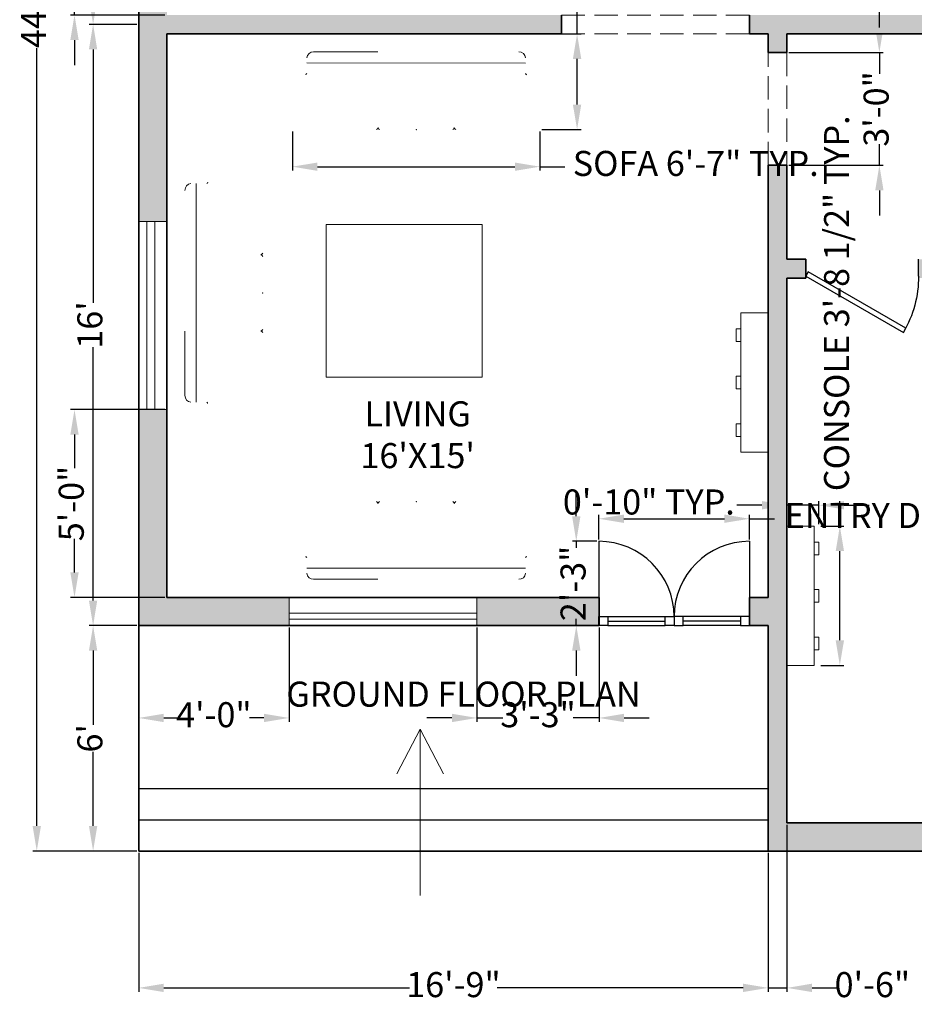
# Model space of a CAD drawing. Units: inches. Extents: x 2073 to 2646, y 2372 to 3017.
# Tile 1 of 8: x 2110 to 2396, y 2372 to 2686. Entities that reach past the tile are written whole.
import ezdxf

# ---------------------------------------------------------------- set-up
doc = ezdxf.new("R2010")
doc.units = ezdxf.units.IN
doc.linetypes.add('DASH', pattern=[0.35, 0.25, -0.1])
for name, color, linetype, lineweight in [('A-ANNO-DIMS', 2, 'Continuous', 18), ('A-ANNO-SYMB', 7, 'Continuous', 18), ('A-ANNO-TEXT', 7, 'Continuous', 25), ('A-AREA-IDEN', 7, 'Continuous', 25), ('A-DOOR', 3, 'Continuous', 25), ('A-FLOR-STRS', 7, 'Continuous', 25), ('A-FURN', 8, 'Continuous', 18), ('A-GLAZ', 4, 'Continuous', 18), ('A-WALL', 7, 'Continuous', 35), ('A-WALL-OVHD', 7, 'DASH', 18), ('A-WALL-PATT', 30, 'Continuous', 13)]:
    doc.layers.add(name, color=color, linetype=linetype, lineweight=lineweight)
doc.styles.get("Standard").update_dxf_attribs({"font": 'arial.ttf'})
doc.dimstyles.new('ISO-25', dxfattribs={"dimtxt": 8, "dimasz": 8, "dimexe": 1.25, "dimexo": 0.625, "dimtad": 0, "dimdec": 1, "dimlunit": 4, "dimtxsty": 'Standard', "dimcen": 2.5, "dimadec": 0, "dimazin": 0, "dimtfac": 1, "dimtdec": 1, "dimtmove": 0, "dimatfit": 3, "dimfxl": 1, "dimarcsym": 0})

# ---------------------------------------------------------------- blocks, each defined once
blk = doc.blocks.new('*D1')
at = {"layer": 'A-ANNO-DIMS', "color": 0, "lineweight": -2, "transparency": 16777216}
for p, q in [((2147.67, 2492.66), (2132.48, 2492.66)), ((2133.73, 2484.66), (2133.73, 2460.99)), ((2133.73, 2428.66), (2133.73, 2452.34)), ((2147.67, 2420.66), (2132.48, 2420.66))]:
    blk.add_line(p, q, dxfattribs=at)
at = {"layer": 'A-ANNO-DIMS', "color": 0, "transparency": 16777216}
for points in [[(2132.4, 2484.66), (2135.06, 2484.66), (2133.73, 2492.66)], [(2132.4, 2428.66), (2135.06, 2428.66), (2133.73, 2420.66)]]:
    blk.add_solid(points, dxfattribs=at)
at = {"layer": 'Defpoints', "color": 0, "transparency": 16777216}
for p in [(2133.73, 2492.66), (2148.29, 2492.66), (2148.29, 2420.66)]:
    blk.add_point(p, dxfattribs=at)
at = {"layer": 'A-ANNO-DIMS', "color": 0, "transparency": 16777216, "insert": (2133.73, 2456.66), "char_height": 8, "attachment_point": 5, "rotation": 90}
blk.add_mtext("6'", dxfattribs=at)
blk = doc.blocks.new('*D2')
at = {"layer": 'A-ANNO-DIMS', "color": 0, "lineweight": -2, "transparency": 16777216}
for p, q in [((2147.67, 2684.66), (2132.48, 2684.66)), ((2133.73, 2676.66), (2133.73, 2595.7)), ((2133.73, 2500.66), (2133.73, 2581.63)), ((2147.67, 2492.66), (2132.48, 2492.66))]:
    blk.add_line(p, q, dxfattribs=at)
at = {"layer": 'A-ANNO-DIMS', "color": 0, "transparency": 16777216}
for points in [[(2132.4, 2676.66), (2135.06, 2676.66), (2133.73, 2684.66)], [(2132.4, 2500.66), (2135.06, 2500.66), (2133.73, 2492.66)]]:
    blk.add_solid(points, dxfattribs=at)
at = {"layer": 'Defpoints', "color": 0, "transparency": 16777216}
for p in [(2133.73, 2684.66), (2148.29, 2684.66), (2148.29, 2492.66)]:
    blk.add_point(p, dxfattribs=at)
at = {"layer": 'A-ANNO-DIMS', "color": 0, "transparency": 16777216, "insert": (2133.73, 2588.66), "char_height": 8, "attachment_point": 5, "rotation": 90}
blk.add_mtext("16'", dxfattribs=at)
blk = doc.blocks.new('*D3')
at = {"layer": 'A-ANNO-DIMS', "color": 0, "lineweight": -2, "transparency": 16777216}
for p, q in [((2147.67, 2948.66), (2132.48, 2948.66)), ((2133.73, 2940.66), (2133.73, 2824.15)), ((2133.73, 2692.66), (2133.73, 2809.18)), ((2147.67, 2684.66), (2132.48, 2684.66))]:
    blk.add_line(p, q, dxfattribs=at)
at = {"layer": 'A-ANNO-DIMS', "color": 0, "transparency": 16777216}
for points in [[(2132.4, 2940.66), (2135.06, 2940.66), (2133.73, 2948.66)], [(2132.4, 2692.66), (2135.06, 2692.66), (2133.73, 2684.66)]]:
    blk.add_solid(points, dxfattribs=at)
at = {"layer": 'Defpoints', "color": 0, "transparency": 16777216}
for p in [(2133.73, 2948.66), (2148.29, 2948.66), (2148.29, 2684.66)]:
    blk.add_point(p, dxfattribs=at)
at = {"layer": 'A-ANNO-DIMS', "color": 0, "transparency": 16777216, "insert": (2133.73, 2816.66), "char_height": 8, "attachment_point": 5, "rotation": 90}
blk.add_mtext("22'", dxfattribs=at)
blk = doc.blocks.new('*D8')
at = {"layer": 'A-ANNO-DIMS', "color": 0, "lineweight": -2, "transparency": 16777216}
for p, q in [((2147.67, 2948.66), (2114.49, 2948.66)), ((2115.74, 2940.66), (2115.74, 2692.24)), ((2115.74, 2428.66), (2115.74, 2677.09)), ((2147.67, 2420.66), (2114.49, 2420.66))]:
    blk.add_line(p, q, dxfattribs=at)
at = {"layer": 'A-ANNO-DIMS', "color": 0, "transparency": 16777216}
for points in [[(2114.41, 2940.66), (2117.08, 2940.66), (2115.74, 2948.66)], [(2114.41, 2428.66), (2117.08, 2428.66), (2115.74, 2420.66)]]:
    blk.add_solid(points, dxfattribs=at)
at = {"layer": 'Defpoints', "color": 0, "transparency": 16777216}
for p in [(2148.29, 2948.66), (2115.74, 2420.66), (2148.29, 2420.66)]:
    blk.add_point(p, dxfattribs=at)
at = {"layer": 'A-ANNO-DIMS', "color": 0, "transparency": 16777216, "insert": (2115.74, 2684.66), "char_height": 8, "attachment_point": 5, "rotation": 90}
blk.add_mtext("44'", dxfattribs=at)
blk = doc.blocks.new('Clinicians and patient chairs 9_dwgmodels.com')
at = {"color": 0}
for points in [[(-907.9, 0, 0, 0, 0), (-959.6, -11.1, 4.62, 4.62, 0)], [(907.9, 0, 0, 0, 0), (-907.9, 0, 4.62, 4.62, 0)], [(959.6, -11.1, 0, 0, 0), (907.9, 0, 4.62, 4.62, 0)], [(-1015.6, -68.3, 0, 0, 0), (-1025.5, -106.3, 4.62, 4.62, 0)], [(-994.7, -35.9, 0, 0, 0), (-1015.6, -68.3, 4.62, 4.62, 0)], [(-959.6, -11.1, 0, 0, 0), (-994.7, -35.9, 4.62, 4.62, 0)], [(994.7, -35.9, 0, 0, 0), (959.6, -11.1, 4.62, 4.62, 0)], [(1015.6, -68.3, 0, 0, 0), (994.7, -35.9, 4.62, 4.62, 0)], [(1025.5, -106.3, 0, 0, 0), (1015.6, -68.3, 4.62, 4.62, 0)], [(-1025.5, -106.3, 0, 0, 0), (-1025.5, -779.5, 4.62, 4.62, 0)], [(-313.4, -149.9, 0, 0, 0), (-318.1, -149.9, 4.62, 4.62, 0)], [(-314.5, -150.4, 0, 0, 0), (-315.7, -159.3, 4.62, 4.62, 0)], [(-315.7, -159.3, 0, 0, 0), (-315.7, -777.3, 4.62, 4.62, 0)], [(-309.5, -148.3, 0, 0, 0), (-314.5, -150.4, 4.62, 4.62, 0)], [(-308, -148.3, 0, 0, 0), (-309.5, -148.3, 4.62, 4.62, 0)], [(-307.5, -148.3, 0, 0, 0), (-308, -148.3, 4.62, 4.62, 0)], [(242.9, -148.3, 0, 0, 0), (-307.5, -148.3, 4.62, 4.62, 0)], [(242.9, -148.3, 0, 0, 0), (296, -148.3, 4.62, 4.62, 0)], [(296, -148.3, 0, 0, 0), (307.5, -148.3, 4.62, 4.62, 0)], [(308, -148.3, 0, 0, 0), (307.5, -148.3, 4.62, 4.62, 0)], [(309.5, -148.3, 0, 0, 0), (308, -148.3, 4.62, 4.62, 0)], [(309.5, -148.3, 0, 0, 0), (314.5, -150.4, 4.62, 4.62, 0)], [(849.5, -149.9, 0, 0, 0), (313.4, -149.9, 4.62, 4.62, 0)], [(314.5, -150.4, 0, 0, 0), (315.7, -159.3, 4.62, 4.62, 0)], [(315.7, -159.3, 0, 0, 0), (315.7, -777.3, 4.62, 4.62, 0)], [(315.7, -161.8, 0, 0, 0), (315.7, -777.3, 4.62, 4.62, 0)], [(1025.5, -779.5, 0, 0, 0), (1025.5, -106.3, 4.62, 4.62, 0)], [(1025.5, -779.5, 0, 0, 0), (1025.5, -117.3, 4.62, 4.62, 0)], [(-906.6, -285, 0, 0, 0), (-906.4, -198.1, 4.62, 4.62, 0)], [(906.9, -327, 0, 0, 0), (906.4, -199.7, 4.62, 4.62, 0)], [(-906.8, -305.4, 0, 0, 0), (-906.9, -324.5, 4.62, 4.62, 0)], [(-906.9, -324.5, 0, 0, 0), (-906.9, -329.8, 4.62, 4.62, 0)], [(-906.6, -285, 0, 0, 0), (-906.8, -305.4, 4.62, 4.62, 0)], [(906.9, -327, 0, 0, 0), (906.9, -329.9, 4.62, 4.62, 0)], [(-1023, -329.7, 0, 0, 0), (-1019.2, -332.9, 4.62, 4.62, 0)], [(-1019.8, -340.2, 0, 0, 0), (-1023, -348.6, 4.62, 4.62, 0)], [(-1010.3, -335.9, 0, 0, 0), (-1019.8, -340.2, 4.62, 4.62, 0)], [(-1019.2, -332.9, 0, 0, 0), (-1019, -333, 4.62, 4.62, 0)], [(-1019, -333, 0, 0, 0), (-1018.9, -333.1, 4.62, 4.62, 0)], [(-1013.9, -334.2, 0, 0, 0), (-1018.9, -333.1, 4.62, 4.62, 0)], [(-1013.9, -334.2, 0, 0, 0), (-964.4, -335.7, 4.62, 4.62, 0)], [(-917.1, -337, 0, 0, 0), (-1010.3, -335.9, 4.62, 4.62, 0)], [(-964.4, -335.7, 0, 0, 0), (-927.1, -336.8, 4.62, 4.62, 0)], [(964.4, -335.7, 0, 0, 0), (914.9, -337.2, 4.62, 4.62, 0)], [(917.1, -339.4, 0, 0, 0), (1010.3, -338.4, 4.62, 4.62, 0)], [(1013.9, -334.2, 0, 0, 0), (964.4, -335.7, 4.62, 4.62, 0)], [(1010.3, -338.4, 0, 0, 0), (1019.8, -342.7, 4.62, 4.62, 0)], [(1013.9, -334.2, 0, 0, 0), (1018.9, -333.1, 4.62, 4.62, 0)], [(1018.9, -333.1, 0, 0, 0), (1019, -333, 4.62, 4.62, 0)], [(1019.2, -332.9, 0, 0, 0), (1019, -333, 4.62, 4.62, 0)], [(1023, -329.7, 0, 0, 0), (1019.2, -332.9, 4.62, 4.62, 0)], [(1019.8, -342.7, 0, 0, 0), (1023, -351.1, 4.62, 4.62, 0)], [(1023, -351.1, 0, 0, 0), (1022.6, -779.8, 4.62, 4.62, 0)], [(-1025.5, -779.5, 0, 0, 0), (-1022.2, -788.7, 4.62, 4.62, 0)], [(-1022.2, -788.7, 0, 0, 0), (-1021.6, -789.8, 4.62, 4.62, 0)], [(-1021.6, -789.8, 0, 0, 0), (-1020.6, -790.5, 4.62, 4.62, 0)], [(-1020.6, -790.5, 0, 0, 0), (-1013.6, -793.7, 4.62, 4.62, 0)], [(-1013.6, -793.7, 0, 0, 0), (1013.6, -793.7, 4.62, 4.62, 0)], [(1019.8, -788.8, 0, 0, 0), (1013.1, -793.7, 4.62, 4.62, 0)], [(1013.6, -793.7, 0, 0, 0), (1020.6, -790.5, 4.62, 4.62, 0)], [(1022.6, -779.8, 0, 0, 0), (1019.8, -788.8, 4.62, 4.62, 0)], [(1020.6, -790.5, 0, 0, 0), (1021.6, -789.8, 4.62, 4.62, 0)], [(1022.2, -788.7, 0, 0, 0), (1021.6, -789.8, 4.62, 4.62, 0)], [(1022.2, -788.7, 0, 0, 0), (1025.5, -779.5, 4.62, 4.62, 0)]]:
    blk.add_lwpolyline(points, format="xyseb", dxfattribs=at)
for points in [[(-849.5, -149.9), (-318.1, -149.9)], [(-906.5, -241.5), (906.5, -242.3)]]:
    blk.add_lwpolyline(points, dxfattribs=at)
for centre, radius, start, end in [((-851.7, -204.8), 54.9, 87.66794, 174.72556), ((851.7, -204.8), 54.9, 5.27444, 92.33206), ((-916.6, -326.8), 10.2, 267.54544, 342.40568), ((916.9, -329.4), 10, 182.60942, 270.79497), ((-337, -773.8), 21.5, 292.11503, 350.63044), ((-294.5, -773.8), 21.5, 189.36956, 247.88497), ((294.5, -773.8), 21.5, 292.11503, 350.63044), ((336.9, -773.8), 21.5, 189.36956, 247.88497)]:
    blk.add_arc(centre, radius, start, end, dxfattribs=at)
blk.add_point((0, -793.7), dxfattribs=at)
blk = doc.blocks.new('*U19')
for p, q in [((0, 0), (0, -6)), ((40, 0), (40, -6))]:
    blk.add_line(p, q)
blk.add_lwpolyline([(0, 0), (34.64, 20), (35.52, 18.48), (0.87, -1.52)], close=True)
blk.add_arc((0, 0), 40, 0, 30)
blk = doc.blocks.new('md')
for points in [[(1926.45, 2847.63), (1926.45, 2824.6)], [(1972.51, 2847.63), (1972.51, 2824.6)], [(1929.2, 2824.6), (1946.72, 2824.6)], [(1969.76, 2824.6), (1952.24, 2824.6)], [(1929.2, 2823.22), (1946.72, 2823.22)], [(1929.2, 2821.85), (1946.72, 2821.85)], [(1969.76, 2823.22), (1952.24, 2823.22)], [(1969.76, 2821.85), (1952.24, 2821.85)]]:
    blk.add_lwpolyline(points)
for points in [[(1926.45, 2824.6), (1929.2, 2824.6), (1929.2, 2821.85), (1926.45, 2821.85)], [(1946.72, 2824.6), (1949.48, 2824.6), (1949.48, 2821.85), (1946.72, 2821.85)], [(1946.72, 2824.6), (1949.48, 2824.6), (1949.48, 2821.85), (1946.72, 2821.85)], [(1952.24, 2824.6), (1949.48, 2824.6), (1949.48, 2821.85), (1952.24, 2821.85)], [(1972.51, 2824.6), (1969.76, 2824.6), (1969.76, 2821.85), (1972.51, 2821.85)]]:
    blk.add_lwpolyline(points, close=True)
for centre, start, end in [((1926.45, 2824.6), 0, 90), ((1972.51, 2824.6), 90, 180)]:
    blk.add_arc(centre, 23.03, start, end)
blk = doc.blocks.new('GLAZ-60IN')
for p, q in [((0, 60), (0, 0)), ((2.6, 60), (2.6, 0))]:
    blk.add_line(p, q)
blk = doc.blocks.new('WALL-CONSOLE-44IN')
for points in [[(10.22, 44.47), (1.5, 44.47), (1.5, 0), (10.22, 0)], [(1.5, 39.34), (0, 39.34), (0, 35.33), (1.5, 35.33)], [(1.5, 24.24), (0, 24.24), (0, 20.23), (1.5, 20.23)], [(1.5, 8.99), (0, 8.99), (0, 4.98), (1.5, 4.98)]]:
    blk.add_lwpolyline(points, close=True)
blk = doc.blocks.new('*D29')
at = {"layer": 'A-ANNO-DIMS', "color": 0, "lineweight": -2, "transparency": 16777216}
for p, q in [((2372.17, 2524.43), (2372.17, 2532.43)), ((2366.13, 2524.43), (2373.42, 2524.43)), ((2372.17, 2487.96), (2372.17, 2516.43)), ((2366.13, 2479.96), (2373.42, 2479.96))]:
    blk.add_line(p, q, dxfattribs=at)
at = {"layer": 'A-ANNO-DIMS', "color": 0, "transparency": 16777216}
for points in [[(2370.84, 2516.43), (2373.51, 2516.43), (2372.17, 2524.43)], [(2370.84, 2487.96), (2373.51, 2487.96), (2372.17, 2479.96)]]:
    blk.add_solid(points, dxfattribs=at)
at = {"layer": 'Defpoints', "color": 0, "transparency": 16777216}
for p in [(2365.5, 2524.43), (2372.17, 2524.43), (2365.5, 2479.96)]:
    blk.add_point(p, dxfattribs=at)
at = {"layer": 'A-ANNO-DIMS', "color": 0, "transparency": 16777216, "insert": (2372.17, 2595.59), "char_height": 8, "attachment_point": 5, "rotation": 90}
blk.add_mtext('CONSOLE 3\'-8 1/2" TYP.', dxfattribs=at)
blk = doc.blocks.new('*D30')
at = {"layer": 'A-ANNO-DIMS', "color": 0, "lineweight": -2, "transparency": 16777216}
for p, q in [((2355.29, 2525.05), (2355.29, 2532.35)), ((2365.5, 2525.05), (2365.5, 2532.35)), ((2347.29, 2531.1), (2339.29, 2531.1)), ((2365.5, 2531.1), (2355.29, 2531.1)), ((2373.5, 2531.1), (2381.5, 2531.1))]:
    blk.add_line(p, q, dxfattribs=at)
at = {"layer": 'A-ANNO-DIMS', "color": 0, "transparency": 16777216}
for points in [[(2347.29, 2532.43), (2347.29, 2529.77), (2355.29, 2531.1)], [(2373.5, 2532.43), (2373.5, 2529.77), (2365.5, 2531.1)]]:
    blk.add_solid(points, dxfattribs=at)
at = {"layer": 'Defpoints', "color": 0, "transparency": 16777216}
for p in [(2355.29, 2531.1), (2355.29, 2524.43), (2365.5, 2524.43)]:
    blk.add_point(p, dxfattribs=at)
at = {"layer": 'A-ANNO-DIMS', "color": 0, "transparency": 16777216, "insert": (2311.18, 2531.1), "char_height": 8, "attachment_point": 5}
blk.add_mtext('0\'-10" TYP.', dxfattribs=at)
blk = doc.blocks.new('*D31')
at = {"layer": 'A-ANNO-DIMS', "color": 0, "lineweight": -2, "transparency": 16777216}
for p, q in [((2197.36, 2650.45), (2197.36, 2637.97)), ((2276.41, 2650.45), (2276.41, 2637.97)), ((2205.36, 2639.22), (2268.41, 2639.22)), ((2276.41, 2639.22), (2284.41, 2639.22))]:
    blk.add_line(p, q, dxfattribs=at)
at = {"layer": 'A-ANNO-DIMS', "color": 0, "transparency": 16777216}
for points in [[(2205.36, 2640.55), (2205.36, 2637.88), (2197.36, 2639.22)], [(2268.41, 2640.55), (2268.41, 2637.88), (2276.41, 2639.22)]]:
    blk.add_solid(points, dxfattribs=at)
at = {"layer": 'Defpoints', "color": 0, "transparency": 16777216}
for p in [(2197.36, 2651.07), (2276.41, 2651.07), (2276.41, 2639.22)]:
    blk.add_point(p, dxfattribs=at)
at = {"layer": 'A-ANNO-DIMS', "color": 0, "transparency": 16777216, "insert": (2326.16, 2639.22), "char_height": 8, "attachment_point": 5}
blk.add_mtext('SOFA 6\'-7" TYP.', dxfattribs=at)
blk = doc.blocks.new('*D32')
at = {"layer": 'A-ANNO-DIMS', "color": 0, "lineweight": -2, "transparency": 16777216}
for p, q in [((2288.27, 2681.66), (2288.27, 2689.66)), ((2277.03, 2681.66), (2289.52, 2681.66)), ((2288.27, 2659.07), (2288.27, 2673.66)), ((2277.03, 2651.07), (2289.52, 2651.07))]:
    blk.add_line(p, q, dxfattribs=at)
at = {"layer": 'A-ANNO-DIMS', "color": 0, "transparency": 16777216}
for points in [[(2286.93, 2673.66), (2289.6, 2673.66), (2288.27, 2681.66)], [(2286.93, 2659.07), (2289.6, 2659.07), (2288.27, 2651.07)]]:
    blk.add_solid(points, dxfattribs=at)
at = {"layer": 'Defpoints', "color": 0, "transparency": 16777216}
for p in [(2276.41, 2681.66), (2288.27, 2681.66), (2276.41, 2651.07)]:
    blk.add_point(p, dxfattribs=at)
at = {"layer": 'A-ANNO-DIMS', "color": 0, "transparency": 16777216, "insert": (2288.27, 2724.06), "char_height": 8, "attachment_point": 5, "rotation": 90}
blk.add_mtext('2\'-6 1/2" TYP.', dxfattribs=at)
blk = doc.blocks.new('*D41')
at = {"layer": 'A-ANNO-DIMS', "color": 0, "lineweight": -2, "transparency": 16777216}
for p, q in [((2295.23, 2520.2), (2295.23, 2528.03)), ((2303.23, 2526.78), (2335.29, 2526.78)), ((2343.29, 2520.2), (2343.29, 2528.03)), ((2343.29, 2526.78), (2351.29, 2526.78))]:
    blk.add_line(p, q, dxfattribs=at)
at = {"layer": 'A-ANNO-DIMS', "color": 0, "transparency": 16777216}
for points in [[(2303.23, 2528.12), (2303.23, 2525.45), (2295.23, 2526.78)], [(2335.29, 2528.12), (2335.29, 2525.45), (2343.29, 2526.78)]]:
    blk.add_solid(points, dxfattribs=at)
at = {"layer": 'Defpoints', "color": 0, "transparency": 16777216}
for p in [(2343.29, 2526.78), (2295.23, 2519.57), (2343.29, 2519.57)]:
    blk.add_point(p, dxfattribs=at)
at = {"layer": 'A-ANNO-DIMS', "color": 0, "transparency": 16777216, "insert": (2401.15, 2526.78), "char_height": 8, "attachment_point": 5}
blk.add_mtext('ENTRY DOOR 4\'-0"', dxfattribs=at)
blk = doc.blocks.new('*D42')
at = {"layer": 'A-ANNO-DIMS', "color": 0, "lineweight": -2, "transparency": 16777216}
for p, q in [((2288.02, 2527.57), (2288.02, 2535.57)), ((2294.6, 2519.57), (2286.77, 2519.57)), ((2288.02, 2519.57), (2288.02, 2517.44)), ((2288.02, 2492.66), (2288.02, 2494.79)), ((2294.6, 2492.66), (2286.77, 2492.66)), ((2288.02, 2484.66), (2288.02, 2476.66))]:
    blk.add_line(p, q, dxfattribs=at)
at = {"layer": 'A-ANNO-DIMS', "color": 0, "transparency": 16777216}
for points in [[(2286.68, 2527.57), (2289.35, 2527.57), (2288.02, 2519.57)], [(2286.68, 2484.66), (2289.35, 2484.66), (2288.02, 2492.66)]]:
    blk.add_solid(points, dxfattribs=at)
at = {"layer": 'Defpoints', "color": 0, "transparency": 16777216}
for p in [(2288.02, 2519.57), (2295.23, 2519.57), (2295.23, 2492.66)]:
    blk.add_point(p, dxfattribs=at)
at = {"layer": 'A-ANNO-DIMS', "color": 0, "transparency": 16777216, "insert": (2288.02, 2506.12), "char_height": 8, "attachment_point": 5, "rotation": 90}
blk.add_mtext('2\'-3"', dxfattribs=at)
blk = doc.blocks.new('*D43')
at = {"layer": 'A-ANNO-DIMS', "color": 0, "lineweight": -2, "transparency": 16777216}
for p, q in [((2148.29, 2420.04), (2148.29, 2375.7)), ((2349.29, 2420.04), (2349.29, 2375.7)), ((2156.29, 2376.95), (2234.8, 2376.95)), ((2341.29, 2376.95), (2262.78, 2376.95))]:
    blk.add_line(p, q, dxfattribs=at)
at = {"layer": 'A-ANNO-DIMS', "color": 0, "transparency": 16777216}
for points in [[(2156.29, 2378.29), (2156.29, 2375.62), (2148.29, 2376.95)], [(2341.29, 2378.29), (2341.29, 2375.62), (2349.29, 2376.95)]]:
    blk.add_solid(points, dxfattribs=at)
at = {"layer": 'Defpoints', "color": 0, "transparency": 16777216}
for p in [(2148.29, 2420.66), (2349.29, 2420.66), (2349.29, 2376.95)]:
    blk.add_point(p, dxfattribs=at)
at = {"layer": 'A-ANNO-DIMS', "color": 0, "transparency": 16777216, "insert": (2248.79, 2376.95), "char_height": 8, "attachment_point": 5}
blk.add_mtext('16\'-9"', dxfattribs=at)
blk = doc.blocks.new('*D47')
at = {"layer": 'A-ANNO-DIMS', "color": 0, "lineweight": -2, "transparency": 16777216}
for p, q in [((2355.29, 2429.04), (2355.29, 2375.7)), ((2349.29, 2420.04), (2349.29, 2375.7)), ((2341.29, 2376.95), (2333.29, 2376.95)), ((2349.29, 2376.95), (2355.29, 2376.95)), ((2363.29, 2376.95), (2371.29, 2376.95))]:
    blk.add_line(p, q, dxfattribs=at)
at = {"layer": 'A-ANNO-DIMS', "color": 0, "transparency": 16777216}
for points in [[(2341.29, 2378.29), (2341.29, 2375.62), (2349.29, 2376.95)], [(2363.29, 2378.29), (2363.29, 2375.62), (2355.29, 2376.95)]]:
    blk.add_solid(points, dxfattribs=at)
at = {"layer": 'Defpoints', "color": 0, "transparency": 16777216}
for p in [(2355.29, 2429.66), (2349.29, 2420.66), (2355.29, 2376.95)]:
    blk.add_point(p, dxfattribs=at)
at = {"layer": 'A-ANNO-DIMS', "color": 0, "transparency": 16777216, "insert": (2382.55, 2376.95), "char_height": 8, "attachment_point": 5}
blk.add_mtext('0\'-6"', dxfattribs=at)
blk = doc.blocks.new('*D48')
at = {"layer": 'A-ANNO-DIMS', "color": 0, "lineweight": -2, "transparency": 16777216}
for p, q in [((2148.29, 2492.04), (2148.29, 2461.91)), ((2196.29, 2492.04), (2196.29, 2461.91)), ((2156.29, 2463.16), (2160.87, 2463.16)), ((2188.29, 2463.16), (2183.71, 2463.16))]:
    blk.add_line(p, q, dxfattribs=at)
at = {"layer": 'A-ANNO-DIMS', "color": 0, "transparency": 16777216}
for points in [[(2156.29, 2464.5), (2156.29, 2461.83), (2148.29, 2463.16)], [(2188.29, 2464.5), (2188.29, 2461.83), (2196.29, 2463.16)]]:
    blk.add_solid(points, dxfattribs=at)
at = {"layer": 'Defpoints', "color": 0, "transparency": 16777216}
for p in [(2148.29, 2492.66), (2196.29, 2492.66), (2148.29, 2463.16)]:
    blk.add_point(p, dxfattribs=at)
at = {"layer": 'A-ANNO-DIMS', "color": 0, "transparency": 16777216, "insert": (2172.29, 2463.16), "char_height": 8, "attachment_point": 5}
blk.add_mtext('4\'-0"', dxfattribs=at)
blk = doc.blocks.new('*D49')
at = {"layer": 'A-ANNO-DIMS', "color": 0, "lineweight": -2, "transparency": 16777216}
for p, q in [((2256.29, 2492.04), (2256.29, 2461.91)), ((2295.29, 2492.04), (2295.29, 2461.91)), ((2248.29, 2463.16), (2240.29, 2463.16)), ((2256.29, 2463.16), (2264.53, 2463.16)), ((2295.29, 2463.16), (2287.05, 2463.16)), ((2303.29, 2463.16), (2311.29, 2463.16))]:
    blk.add_line(p, q, dxfattribs=at)
at = {"layer": 'A-ANNO-DIMS', "color": 0, "transparency": 16777216}
for points in [[(2248.29, 2464.5), (2248.29, 2461.83), (2256.29, 2463.16)], [(2303.29, 2464.5), (2303.29, 2461.83), (2295.29, 2463.16)]]:
    blk.add_solid(points, dxfattribs=at)
at = {"layer": 'Defpoints', "color": 0, "transparency": 16777216}
for p in [(2256.29, 2492.66), (2295.29, 2492.66), (2256.29, 2463.16)]:
    blk.add_point(p, dxfattribs=at)
at = {"layer": 'A-ANNO-DIMS', "color": 0, "transparency": 16777216, "insert": (2275.79, 2463.16), "char_height": 8, "attachment_point": 5}
blk.add_mtext('3\'-3"', dxfattribs=at)
blk = doc.blocks.new('*D53')
at = {"layer": 'A-ANNO-DIMS', "color": 0, "lineweight": -2, "transparency": 16777216}
for p, q in [((2384.79, 2683.66), (2384.79, 2691.66)), ((2355.92, 2675.66), (2386.04, 2675.66)), ((2384.79, 2675.66), (2384.79, 2668.92)), ((2384.79, 2639.66), (2384.79, 2646.41)), ((2355.92, 2639.66), (2386.04, 2639.66)), ((2384.79, 2631.66), (2384.79, 2623.66))]:
    blk.add_line(p, q, dxfattribs=at)
at = {"layer": 'A-ANNO-DIMS', "color": 0, "transparency": 16777216}
for points in [[(2383.46, 2683.66), (2386.12, 2683.66), (2384.79, 2675.66)], [(2383.46, 2631.66), (2386.12, 2631.66), (2384.79, 2639.66)]]:
    blk.add_solid(points, dxfattribs=at)
at = {"layer": 'Defpoints', "color": 0, "transparency": 16777216}
for p in [(2355.29, 2675.66), (2355.29, 2639.66), (2384.79, 2639.66)]:
    blk.add_point(p, dxfattribs=at)
at = {"layer": 'A-ANNO-DIMS', "color": 0, "transparency": 16777216, "insert": (2384.79, 2657.66), "char_height": 8, "attachment_point": 5, "rotation": 90}
blk.add_mtext('3\'-0"', dxfattribs=at)
blk = doc.blocks.new('*D59')
at = {"layer": 'A-ANNO-DIMS', "color": 0, "lineweight": -2, "transparency": 16777216}
for p, q in [((2156.67, 2561.66), (2126.54, 2561.66)), ((2127.79, 2553.66), (2127.79, 2542.92)), ((2127.79, 2509.66), (2127.79, 2520.41)), ((2156.67, 2501.66), (2126.54, 2501.66))]:
    blk.add_line(p, q, dxfattribs=at)
at = {"layer": 'A-ANNO-DIMS', "color": 0, "transparency": 16777216}
for points in [[(2126.46, 2553.66), (2129.12, 2553.66), (2127.79, 2561.66)], [(2126.46, 2509.66), (2129.12, 2509.66), (2127.79, 2501.66)]]:
    blk.add_solid(points, dxfattribs=at)
at = {"layer": 'Defpoints', "color": 0, "transparency": 16777216}
for p in [(2127.79, 2561.66), (2157.29, 2561.66), (2157.29, 2501.66)]:
    blk.add_point(p, dxfattribs=at)
at = {"layer": 'A-ANNO-DIMS', "color": 0, "transparency": 16777216, "insert": (2127.79, 2531.66), "char_height": 8, "attachment_point": 5, "rotation": 90}
blk.add_mtext('5\'-0"', dxfattribs=at)
blk = doc.blocks.new('*D60')
at = {"layer": 'A-ANNO-DIMS', "color": 0, "lineweight": -2, "transparency": 16777216}
for p, q in [((2127.79, 2712.25), (2127.79, 2720.25)), ((2156.67, 2704.25), (2126.54, 2704.25)), ((2127.79, 2687.66), (2127.79, 2704.25)), ((2156.67, 2687.66), (2126.54, 2687.66)), ((2127.79, 2679.66), (2127.79, 2671.66))]:
    blk.add_line(p, q, dxfattribs=at)
at = {"layer": 'A-ANNO-DIMS', "color": 0, "transparency": 16777216}
for points in [[(2126.46, 2712.25), (2129.12, 2712.25), (2127.79, 2704.25)], [(2126.46, 2679.66), (2129.12, 2679.66), (2127.79, 2687.66)]]:
    blk.add_solid(points, dxfattribs=at)
at = {"layer": 'Defpoints', "color": 0, "transparency": 16777216}
for p in [(2127.79, 2704.25), (2157.29, 2704.25), (2157.29, 2687.66)]:
    blk.add_point(p, dxfattribs=at)
at = {"layer": 'A-ANNO-DIMS', "color": 0, "transparency": 16777216, "insert": (2127.79, 2740.45), "char_height": 8, "attachment_point": 5, "rotation": 90}
blk.add_mtext('1\'-4 1/2"', dxfattribs=at)

msp = doc.modelspace()

# ---------------------------------------------------------------- hatches: boundary and pattern name
at = {"layer": 'A-WALL-PATT'}
h = msp.add_hatch(color=256, dxfattribs=at)
h.dxf.hatch_style = 1
h.paths.add_polyline_path([(2340.29, 2948.66), (2148.29, 2948.66), (2148.29, 2924.66), (2157.29, 2924.66), (2157.29, 2939.66), (2313.29, 2939.66), (2313.29, 2885.66), (2307.29, 2885.66), (2307.29, 2879.66), (2313.29, 2879.66), (2313.29, 2777.66), (2319.29, 2777.66), (2319.29, 2831.66), (2385.29, 2831.66), (2385.29, 2825.68), (2390.69, 2825.68, -0.004149), (2391.29, 2825.68), (2391.29, 2843.66), (2385.29, 2843.66), (2385.29, 2837.66), (2319.29, 2837.66), (2319.29, 2939.66), (2340.29, 2939.66)])
h.paths.add_polyline_path([(2271.29, 2885.66), (2157.29, 2885.66), (2157.29, 2900.66), (2148.29, 2900.66), (2148.29, 2856.74), (2157.29, 2856.74), (2157.29, 2879.66), (2271.29, 2879.66)], flags=17)
h.paths.add_polyline_path([(2157.29, 2796.74), (2148.29, 2796.74), (2148.29, 2764.25), (2157.29, 2764.25)])
h.paths.add_polyline_path([(2157.29, 2681.66), (2283.29, 2681.66), (2283.29, 2687.66), (2157.29, 2687.66), (2157.29, 2704.25), (2148.29, 2704.25), (2148.29, 2621.66), (2157.29, 2621.66)])
h.paths.add_polyline_path([(2196.29, 2501.66), (2157.29, 2501.66), (2157.29, 2561.66), (2148.29, 2561.66), (2148.29, 2492.66), (2196.29, 2492.66)])
h.paths.add_polyline_path([(2295.23, 2495.54), (2295.23, 2501.66), (2256.29, 2501.66), (2256.29, 2492.66), (2295.23, 2492.66)])
h.paths.add_polyline_path([(2355.29, 2603.66), (2361.29, 2603.66), (2361.29, 2609.66), (2355.29, 2609.66), (2355.29, 2639.66), (2349.29, 2639.66), (2349.29, 2501.66), (2343.29, 2501.66), (2343.29, 2492.66), (2349.29, 2492.66), (2349.29, 2420.66), (2532.29, 2420.66), (2532.29, 2486.66), (2523.29, 2486.66), (2523.29, 2429.66), (2355.29, 2429.66)])
h.paths.add_polyline_path([(2532.29, 2633.66), (2523.29, 2633.66), (2523.29, 2609.66), (2439.29, 2609.66), (2439.29, 2615.66), (2433.29, 2615.66), (2433.29, 2609.66), (2397.31, 2609.66), (2397.31, 2604.26, -0.004149), (2397.3, 2603.66), (2523.29, 2603.66), (2523.29, 2546.66), (2532.29, 2546.66)], flags=17)
h.paths.add_polyline_path([(2532.29, 2702.66), (2523.29, 2702.66), (2523.29, 2687.66), (2385.29, 2687.66), (2343.29, 2687.66), (2343.29, 2681.66), (2349.29, 2681.66), (2349.29, 2675.66), (2355.29, 2675.66), (2355.29, 2681.66), (2433.29, 2681.66), (2433.29, 2645.66), (2439.29, 2645.66), (2439.29, 2681.66), (2523.29, 2681.66), (2523.29, 2657.66), (2532.29, 2657.66)])
h.paths.add_polyline_path([(2532.29, 2831.66), (2523.29, 2831.66), (2523.29, 2783.66), (2391.29, 2783.66), (2391.29, 2789.66), (2385.29, 2789.66), (2385.29, 2777.66), (2523.29, 2777.66), (2523.29, 2762.66), (2532.29, 2762.66)])
h.paths.add_polyline_path([(2532.29, 2948.66), (2364.29, 2948.66), (2364.29, 2939.66), (2385.29, 2939.66), (2385.29, 2873.66), (2391.29, 2873.66), (2391.29, 2939.66), (2523.29, 2939.66), (2523.29, 2891.66), (2532.29, 2891.66)])

# ---------------------------------------------------------------- linework, layer by layer
at = {"layer": 'A-ANNO-SYMB'}
for p, q in [((2238.15, 2459.56), (2230.68, 2445.29)), ((2238.15, 2406.45), (2238.15, 2459.56)), ((2238.15, 2459.56), (2245.62, 2445.29))]:
    msp.add_line(p, q, dxfattribs=at)
at = {"layer": 'A-FLOR-STRS'}
for p, q in [((2148.29, 2440.66), (2349.29, 2440.66)), ((2148.29, 2430.66), (2349.29, 2430.66))]:
    msp.add_line(p, q, dxfattribs=at)
at = {"layer": 'A-FURN'}
msp.add_lwpolyline([(2208.2, 2620.73), (2257.95, 2620.73), (2257.95, 2572.02), (2208.2, 2572.02)], close=True, dxfattribs=at)
at = {"layer": 'A-GLAZ'}
for p, q in [((2157.29, 2621.66), (2148.29, 2621.66)), ((2157.29, 2561.66), (2148.29, 2561.66)), ((2196.29, 2501.66), (2196.29, 2492.66)), ((2256.29, 2501.66), (2256.29, 2492.66)), ((2196.29, 2496.66), (2256.29, 2496.66)), ((2196.29, 2494.66), (2256.29, 2494.66))]:
    msp.add_line(p, q, dxfattribs=at)
at = {"layer": 'A-WALL'}
for p, q in [((2148.29, 2948.66), (2148.29, 2420.66)), ((2283.29, 2687.66), (2283.29, 2681.66)), ((2343.29, 2687.66), (2343.29, 2681.66)), ((2157.29, 2681.66), (2283.29, 2681.66)), ((2157.29, 2681.66), (2157.29, 2501.66)), ((2343.29, 2681.66), (2349.29, 2681.66)), ((2349.29, 2681.66), (2349.29, 2675.66)), ((2355.29, 2681.66), (2355.29, 2675.66)), ((2355.29, 2681.66), (2433.29, 2681.66)), ((2349.29, 2675.66), (2355.29, 2675.66)), ((2349.29, 2639.66), (2355.29, 2639.66)), ((2349.29, 2639.66), (2349.29, 2501.66)), ((2355.29, 2639.66), (2355.29, 2609.66)), ((2355.29, 2609.66), (2361.29, 2609.66)), ((2361.29, 2609.66), (2361.29, 2603.66)), ((2355.29, 2603.66), (2361.29, 2603.66)), ((2355.29, 2429.66), (2355.29, 2603.66)), ((2157.29, 2501.66), (2295.29, 2501.66)), ((2295.29, 2501.66), (2295.29, 2492.66)), ((2343.29, 2501.66), (2343.29, 2492.66)), ((2343.29, 2501.66), (2349.29, 2501.66)), ((2148.29, 2492.66), (2295.29, 2492.66)), ((2343.29, 2492.66), (2349.29, 2492.66)), ((2349.29, 2492.66), (2349.29, 2420.66)), ((2355.29, 2429.66), (2523.29, 2429.66)), ((2148.29, 2420.66), (2532.29, 2420.66))]:
    msp.add_line(p, q, dxfattribs=at)
at = {"layer": 'A-WALL-OVHD', "ltscale": 30}
for points in [[(2283.29, 2687.66), (2343.29, 2687.66), (2343.29, 2681.66), (2283.29, 2681.66)], [(2349.29, 2675.66), (2355.29, 2675.66), (2355.29, 2639.66), (2349.29, 2639.66)]]:
    msp.add_lwpolyline(points, close=True, dxfattribs=at)

# ---------------------------------------------------------------- block references
at = {"layer": 'A-DOOR', "xscale": -0.90038727397209, "yscale": 0.90038727397209, "zscale": 0.90038727397209, "rotation": 180}
msp.add_blockref('*U19', (2361.29, 2604.26), dxfattribs=at)
at = {"layer": 'A-DOOR', "xscale": 1.043429121125784, "yscale": 1.043429121125784, "zscale": 1.043429121125784}
msp.add_blockref('md', (285.11, -451.73), dxfattribs=at)
at = {"layer": 'A-FURN', "xscale": 0.0385401032590329, "yscale": 0.0385401032590329, "zscale": 0.0385401032590329}
msp.add_blockref('Clinicians and patient chairs 9_dwgmodels.com', (2236.89, 2681.66), dxfattribs=at)
at = {"layer": 'A-FURN', "yscale": 0.0385401032590329, "zscale": 0.0385401032590329}
for p, xscale, rotation in [((2157.29, 2598.91), 0.0385401032590329, 90), ((2236.89, 2501.66), -0.0385401032590329, 180)]:
    msp.add_blockref('Clinicians and patient chairs 9_dwgmodels.com', p, dxfattribs=dict(at, xscale=xscale, rotation=rotation))
at = {"layer": 'A-FURN'}
msp.add_blockref('WALL-CONSOLE-44IN', (2339.07, 2548.07), dxfattribs=at)
at = {"layer": 'A-FURN', "extrusion": (0, 0, -1), "zscale": -1}
msp.add_blockref('WALL-CONSOLE-44IN', (-2365.51, 2479.96), dxfattribs=at)
at = {"layer": 'A-GLAZ'}
msp.add_blockref('GLAZ-60IN', (2150.89, 2561.66), dxfattribs=at)

# ---------------------------------------------------------------- texts
at = {"layer": 'A-ANNO-TEXT', "insert": (2182.04, 2474.77), "char_height": 8, "attachment_point": 1}
msp.add_mtext_dynamic_manual_height_columns('\\pxqc;GROUND FLOOR PLAN', width=139.927, gutter_width=12.5, heights=[0], dxfattribs=at)
at = {"layer": 'A-AREA-IDEN', "insert": (2200.28, 2564.28), "char_height": 8, "attachment_point": 1}
msp.add_mtext_dynamic_manual_height_columns("\\pxqc;LIVING\\P16'X15'", width=74.1792, gutter_width=12.5, heights=[0], dxfattribs=at)

# ---------------------------------------------------------------- dimensions: what is measured, and where the dimension line sits
at = {"layer": 'A-ANNO-DIMS'}
for base, p1, p2, angle, override, picture, middle in [((2115.74, 2420.66), (2148.29, 2948.66), (2148.29, 2420.66), 90, {"dimclrd": 0, "dimclre": 0, "dimclrt": 0}, '*D8', (2115.74, 2684.66)), ((2133.73, 2948.66), (2148.29, 2684.66), (2148.29, 2948.66), 90, {"dimclrd": 0, "dimclre": 0, "dimclrt": 0}, '*D3', (2133.73, 2816.66)), ((2127.79, 2704.25), (2157.29, 2687.66), (2157.29, 2704.25), 90, {"dimdec": 1, "dimlfac": 1, "dimrnd": 0, "dimzin": 1, "dimdsep": 46, "dimlunit": 4, "dimfrac": 2}, '*D60', (2127.79, 2740.45)), ((2384.79, 2639.66), (2355.29, 2675.66), (2355.29, 2639.66), 270, {"dimdec": 1, "dimlfac": 1, "dimrnd": 0, "dimzin": 1, "dimdsep": 46, "dimlunit": 4, "dimfrac": 2}, '*D53', (2384.79, 2657.66)), ((2133.73, 2684.66), (2148.29, 2492.66), (2148.29, 2684.66), 90, {"dimclrd": 0, "dimclre": 0, "dimclrt": 0}, '*D2', (2133.73, 2588.66)), ((2127.79, 2561.66), (2157.29, 2501.66), (2157.29, 2561.66), 90, {"dimdec": 1, "dimlfac": 1, "dimrnd": 0, "dimzin": 1, "dimdsep": 46, "dimlunit": 4, "dimfrac": 2}, '*D59', (2127.79, 2531.66)), ((2288.02, 2519.57), (2295.23, 2492.66), (2295.23, 2519.57), 90, {"dimdec": 1, "dimlfac": 1, "dimrnd": 0, "dimzin": 1, "dimdsep": 46, "dimlunit": 4, "dimfrac": 2}, '*D42', (2288.02, 2506.12)), ((2133.73, 2492.66), (2148.29, 2420.66), (2148.29, 2492.66), 90, {"dimclrd": 0, "dimclre": 0, "dimclrt": 0}, '*D1', (2133.73, 2456.66)), ((2148.29, 2463.16), (2196.29, 2492.66), (2148.29, 2492.66), 180, {"dimdec": 1, "dimlfac": 1, "dimrnd": 0, "dimzin": 1, "dimdsep": 46, "dimlunit": 4, "dimfrac": 2}, '*D48', (2172.29, 2463.16)), ((2256.29, 2463.16), (2295.29, 2492.66), (2256.29, 2492.66), 180, {"dimdec": 1, "dimlfac": 1, "dimrnd": 0, "dimzin": 1, "dimdsep": 46, "dimlunit": 4, "dimfrac": 2}, '*D49', (2275.79, 2463.16))]:
    dim = msp.add_linear_dim(base=base, p1=p1, p2=p2, angle=angle, dimstyle='ISO-25', override=override, dxfattribs=at)
    dim.commit()
    dim.dimension.update_dxf_attribs({"geometry": picture, "text_midpoint": middle})
for base, p1, p2, angle, text, picture, middle in [((2288.27, 2681.66), (2276.41, 2651.07), (2276.41, 2681.66), 90, '<> TYP.', '*D32', (2288.27, 2724.06)), ((2372.17, 2524.43), (2365.5, 2479.96), (2365.5, 2524.43), 90, 'CONSOLE <> TYP.', '*D29', (2372.17, 2595.59)), ((2355.29, 2531.1), (2365.5, 2524.43), (2355.29, 2524.43), 180, '<> TYP.', '*D30', (2311.18, 2531.1))]:
    dim = msp.add_linear_dim(base=base, p1=p1, p2=p2, angle=angle, text=text, dimstyle='ISO-25', override={"dimdec": 1, "dimlfac": 1, "dimrnd": 0, "dimzin": 1, "dimdsep": 46, "dimlunit": 4, "dimfrac": 2}, dxfattribs=at)
    dim.commit()
    dim.dimension.update_dxf_attribs({"geometry": picture, "text_midpoint": middle})
for base, p1, p2, text, picture, middle in [((2276.4094, 2639.2171), (2197.3622, 2651.0742), (2276.4094, 2651.0742), 'SOFA <> TYP.', '*D31', (2326.164, 2639.2171)), ((2343.29, 2526.78), (2295.23, 2519.57), (2343.29, 2519.57), 'ENTRY DOOR <>', '*D41', (2401.15, 2526.78))]:
    dim = msp.add_linear_dim(base=base, p1=p1, p2=p2, text=text, dimstyle='ISO-25', override={"dimdec": 1, "dimlfac": 1, "dimrnd": 0, "dimzin": 1, "dimdsep": 46, "dimlunit": 4, "dimfrac": 2}, dxfattribs=at)
    dim.commit()
    dim.dimension.update_dxf_attribs({"geometry": picture, "text_midpoint": middle})
for base, p1, p2, picture, middle in [((2355.29, 2376.95), (2349.29, 2420.66), (2355.29, 2429.66), '*D47', (2382.55, 2376.95)), ((2349.29, 2376.95), (2148.29, 2420.66), (2349.29, 2420.66), '*D43', (2248.79, 2376.95))]:
    dim = msp.add_linear_dim(base=base, p1=p1, p2=p2, dimstyle='ISO-25', override={"dimdec": 1, "dimlfac": 1, "dimrnd": 0, "dimzin": 1, "dimdsep": 46, "dimlunit": 4, "dimfrac": 2}, dxfattribs=at)
    dim.commit()
    dim.dimension.update_dxf_attribs({"geometry": picture, "text_midpoint": middle})

doc.saveas('drawing.dxf')
